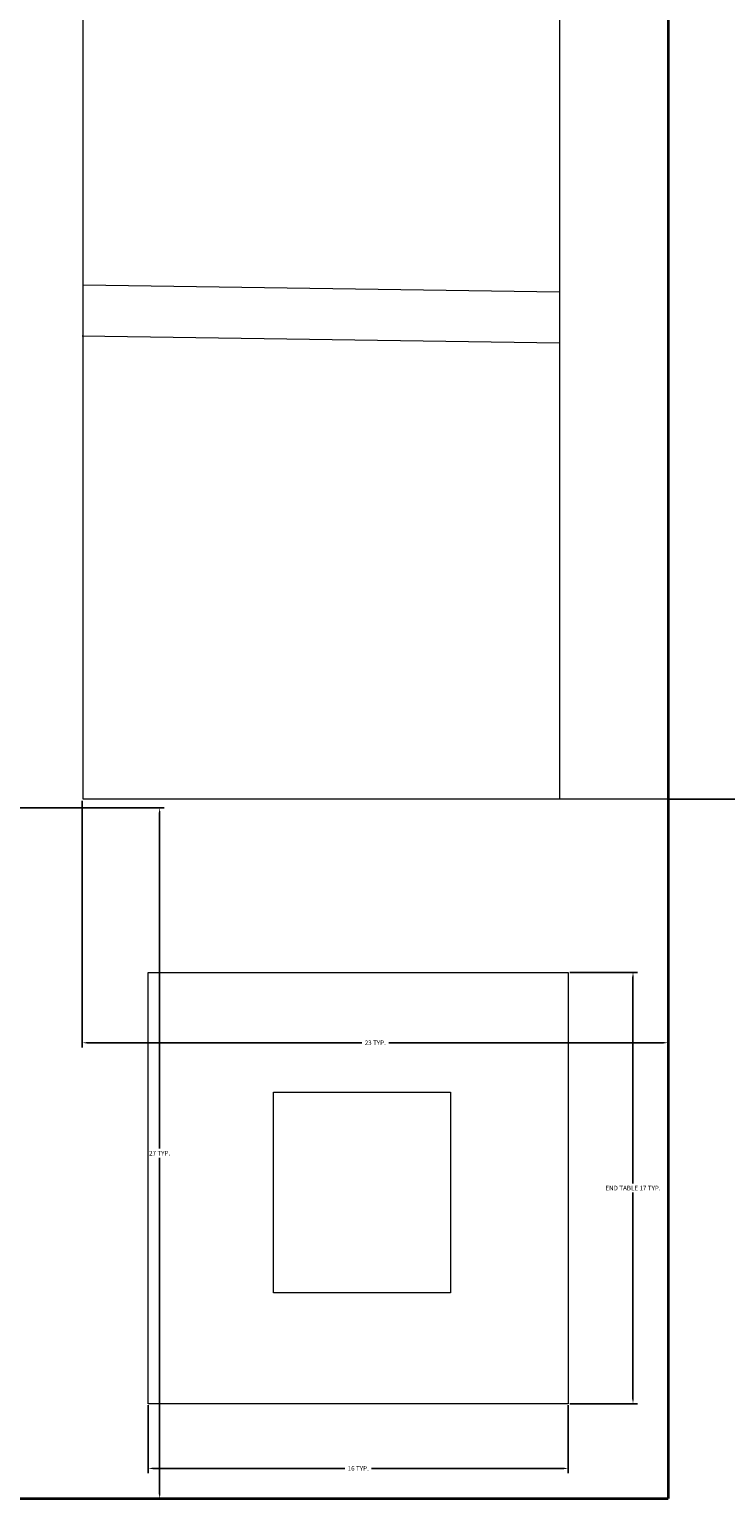
# Model space of a CAD drawing. Units: inches. Extents: x 108 to 613, y 1573 to 2319.
# Tile 6 of 11: x 406 to 434, y 1998 to 2055. Entities that reach past the tile are written whole.
import ezdxf

# ---------------------------------------------------------------- set-up
doc = ezdxf.new("R2010")
doc.units = ezdxf.units.IN
for name, color, linetype, lineweight in [('A-ANNO-DIMS', 2, 'Continuous', 18), ('furniture', 2, 'Continuous', 18), ('wall', 6, 'Continuous', 35)]:
    doc.layers.add(name, color=color, linetype=linetype, lineweight=lineweight)
doc.styles.get("Standard").update_dxf_attribs({"font": 'arial.ttf'})
doc.dimstyles.get("Standard").update_dxf_attribs({"dimtxt": 0.18, "dimasz": 0.18, "dimexe": 0.18, "dimexo": 0.0625, "dimgap": 0.09, "dimtad": 0, "dimtih": 1, "dimtoh": 1, "dimdec": 4, "dimzin": 0, "dimdsep": 46, "dimtxsty": 'Standard', "dimcen": 0.09, "dimadec": 0, "dimazin": 0, "dimtfac": 1, "dimtdec": 4, "dimtofl": 0, "dimtmove": 0, "dimatfit": 3, "dimfxl": 1, "dimtolj": 1, "dimtzin": 0, "dimarcsym": 0})

# ---------------------------------------------------------------- blocks, each defined once
blk = doc.blocks.new('SOFA-3-SEAT')
for p, q in [((18.702, 63.659), (18.702, 0)), ((0.03, 43.076), (18.702, 43.076)), ((0.03, 41.076), (18.702, 41.076)), ((0.03, 20.172), (18.702, 19.893)), ((0, 18.172), (18.702, 17.893))]:
    blk.add_line(p, q)
blk.add_lwpolyline([(0.03, 63.659), (22.965, 63.659), (22.965, 0), (0.03, 0)], close=True)
blk = doc.blocks.new('END-TABLE')
for points in [[(0, 16.912), (16.469, 16.912), (16.469, 0), (0, 0)], [(4.921, 12.212), (11.85, 12.212), (11.85, 4.342), (4.921, 4.342)]]:
    blk.add_lwpolyline(points, close=True)
blk = doc.blocks.new('*D31')
at = {"layer": 'A-ANNO-DIMS', "color": 0, "lineweight": -2, "transparency": 16777216}
for p, q in [((431.338, 2088.692), (441.004, 2088.692)), ((440.824, 2088.512), (440.824, 2057.046)), ((440.824, 2025.213), (440.824, 2056.679)), ((431.338, 2025.033), (441.004, 2025.033))]:
    blk.add_line(p, q, dxfattribs=at)
at = {"layer": 'A-ANNO-DIMS', "color": 0, "transparency": 16777216}
for points in [[(440.794, 2088.512), (440.854, 2088.512), (440.824, 2088.692)], [(440.794, 2025.213), (440.854, 2025.213), (440.824, 2025.033)]]:
    blk.add_solid(points, dxfattribs=at)
at = {"layer": 'Defpoints', "color": 0, "transparency": 16777216}
for p in [(431.275, 2088.692), (440.824, 2088.692), (431.275, 2025.033)]:
    blk.add_point(p, dxfattribs=at)
at = {"layer": 'A-ANNO-DIMS', "color": 0, "transparency": 16777216, "insert": (440.824, 2056.863), "char_height": 0.18, "attachment_point": 5}
blk.add_mtext('\\A1;3-SEAT SOFA 64 TYP.', dxfattribs=at)
blk = doc.blocks.new('*D32')
at = {"layer": 'A-ANNO-DIMS', "color": 0, "lineweight": -2, "transparency": 16777216}
for p, q in [((408.31, 2024.97), (408.31, 2015.304)), ((431.275, 2024.97), (431.275, 2015.304)), ((408.49, 2015.484), (419.263, 2015.484)), ((431.095, 2015.484), (420.322, 2015.484))]:
    blk.add_line(p, q, dxfattribs=at)
at = {"layer": 'A-ANNO-DIMS', "color": 0, "transparency": 16777216}
for points in [[(408.49, 2015.514), (408.49, 2015.454), (408.31, 2015.484)], [(431.095, 2015.514), (431.095, 2015.454), (431.275, 2015.484)]]:
    blk.add_solid(points, dxfattribs=at)
at = {"layer": 'Defpoints', "color": 0, "transparency": 16777216}
for p in [(408.31, 2025.033), (431.275, 2025.033), (431.275, 2015.484)]:
    blk.add_point(p, dxfattribs=at)
at = {"layer": 'A-ANNO-DIMS', "color": 0, "transparency": 16777216, "insert": (419.793, 2015.484), "char_height": 0.18, "attachment_point": 5}
blk.add_mtext('\\A1;23 TYP.', dxfattribs=at)
blk = doc.blocks.new('*D34')
at = {"layer": 'A-ANNO-DIMS', "color": 0, "lineweight": -2, "transparency": 16777216}
for p, q in [((403.006, 2024.696), (411.521, 2024.696)), ((411.341, 2024.516), (411.341, 2011.335)), ((411.341, 1997.792), (411.341, 2010.974)), ((403.006, 1997.612), (411.521, 1997.612))]:
    blk.add_line(p, q, dxfattribs=at)
at = {"layer": 'A-ANNO-DIMS', "color": 0, "transparency": 16777216}
for points in [[(411.311, 2024.516), (411.371, 2024.516), (411.341, 2024.696)], [(411.311, 1997.792), (411.371, 1997.792), (411.341, 1997.612)]]:
    blk.add_solid(points, dxfattribs=at)
at = {"layer": 'Defpoints', "color": 0, "transparency": 16777216}
for p in [(402.944, 2024.696), (411.341, 2024.696), (402.944, 1997.612)]:
    blk.add_point(p, dxfattribs=at)
at = {"layer": 'A-ANNO-DIMS', "color": 0, "transparency": 16777216, "insert": (411.341, 2011.154), "char_height": 0.18, "attachment_point": 5}
blk.add_mtext('\\A1;27 TYP.', dxfattribs=at)
blk = doc.blocks.new('*D35')
at = {"layer": 'A-ANNO-DIMS', "color": 0, "lineweight": -2, "transparency": 16777216}
for p, q in [((427.421, 2018.245), (430.075, 2018.245)), ((429.895, 2018.065), (429.895, 2009.97)), ((429.895, 2001.513), (429.895, 2009.609)), ((427.421, 2001.333), (430.075, 2001.333))]:
    blk.add_line(p, q, dxfattribs=at)
at = {"layer": 'A-ANNO-DIMS', "color": 0, "transparency": 16777216}
for points in [[(429.865, 2018.065), (429.925, 2018.065), (429.895, 2018.245)], [(429.865, 2001.513), (429.925, 2001.513), (429.895, 2001.333)]]:
    blk.add_solid(points, dxfattribs=at)
at = {"layer": 'Defpoints', "color": 0, "transparency": 16777216}
for p in [(427.358, 2018.245), (429.895, 2018.245), (427.358, 2001.333)]:
    blk.add_point(p, dxfattribs=at)
at = {"layer": 'A-ANNO-DIMS', "color": 0, "transparency": 16777216, "insert": (429.895, 2009.789), "char_height": 0.18, "attachment_point": 5}
blk.add_mtext('\\A1;END TABLE 17 TYP.', dxfattribs=at)
blk = doc.blocks.new('*D36')
at = {"layer": 'A-ANNO-DIMS', "color": 0, "lineweight": -2, "transparency": 16777216}
for p, q in [((410.889, 2001.271), (410.889, 1998.616)), ((427.358, 2001.271), (427.358, 1998.616)), ((411.069, 1998.796), (418.604, 1998.796)), ((427.178, 1998.796), (419.643, 1998.796))]:
    blk.add_line(p, q, dxfattribs=at)
at = {"layer": 'A-ANNO-DIMS', "color": 0, "transparency": 16777216}
for points in [[(411.069, 1998.826), (411.069, 1998.766), (410.889, 1998.796)], [(427.178, 1998.826), (427.178, 1998.766), (427.358, 1998.796)]]:
    blk.add_solid(points, dxfattribs=at)
at = {"layer": 'Defpoints', "color": 0, "transparency": 16777216}
for p in [(410.889, 2001.333), (427.358, 2001.333), (427.358, 1998.796)]:
    blk.add_point(p, dxfattribs=at)
at = {"layer": 'A-ANNO-DIMS', "color": 0, "transparency": 16777216, "insert": (419.124, 1998.796), "char_height": 0.18, "attachment_point": 5}
blk.add_mtext('\\A1;16 TYP.', dxfattribs=at)

msp = doc.modelspace()

# ---------------------------------------------------------------- linework, layer by layer
at = {"layer": 'wall'}
for p in [(431.2753, 2092.1125), (341.2753, 1997.6125)]:
    msp.add_line(p, (431.2753, 1997.6125), dxfattribs=at)

# ---------------------------------------------------------------- block references
at = {"layer": 'furniture'}
for name, p in [('SOFA-3-SEAT', (408.31, 2025.033)), ('END-TABLE', (410.889, 2001.333))]:
    msp.add_blockref(name, p, dxfattribs=at)

# ---------------------------------------------------------------- dimensions: what is measured, and where the dimension line sits
at = {"layer": 'A-ANNO-DIMS'}
for base, p1, p2, text, picture, middle in [((440.8243, 2088.6925), (431.2753, 2025.0326), (431.2753, 2088.6925), '3-SEAT SOFA <> TYP.', '*D31', (440.8243, 2056.8625)), ((411.3411, 2024.6958), (402.9438, 1997.6125), (402.9438, 2024.6958), '<> TYP.', '*D34', (411.3411, 2011.1541)), ((429.895, 2018.2452), (427.3582, 2001.3331), (427.3582, 2018.2452), 'END TABLE <> TYP.', '*D35', (429.895, 2009.7891))]:
    dim = msp.add_linear_dim(base=base, p1=p1, p2=p2, angle=90, text=text, dimstyle='Standard', override={"dimdec": 0, "dimlfac": 1, "dimrnd": 0, "dimzin": 0, "dimdsep": 46, "dimlunit": 2}, dxfattribs=at)
    dim.commit()
    dim.dimension.update_dxf_attribs({"geometry": picture, "text_midpoint": middle})
for base, p1, p2, picture, middle in [((431.2753, 2015.4836), (408.3097, 2025.0326), (431.2753, 2025.0326), '*D32', (419.7925, 2015.4836)), ((427.3582, 1998.7963), (410.889, 2001.3331), (427.3582, 2001.3331), '*D36', (419.1236, 1998.7963))]:
    dim = msp.add_linear_dim(base=base, p1=p1, p2=p2, text='<> TYP.', dimstyle='Standard', override={"dimdec": 0, "dimlfac": 1, "dimrnd": 0, "dimzin": 0, "dimdsep": 46, "dimlunit": 2}, dxfattribs=at)
    dim.commit()
    dim.dimension.update_dxf_attribs({"geometry": picture, "text_midpoint": middle})

doc.saveas('drawing.dxf')
